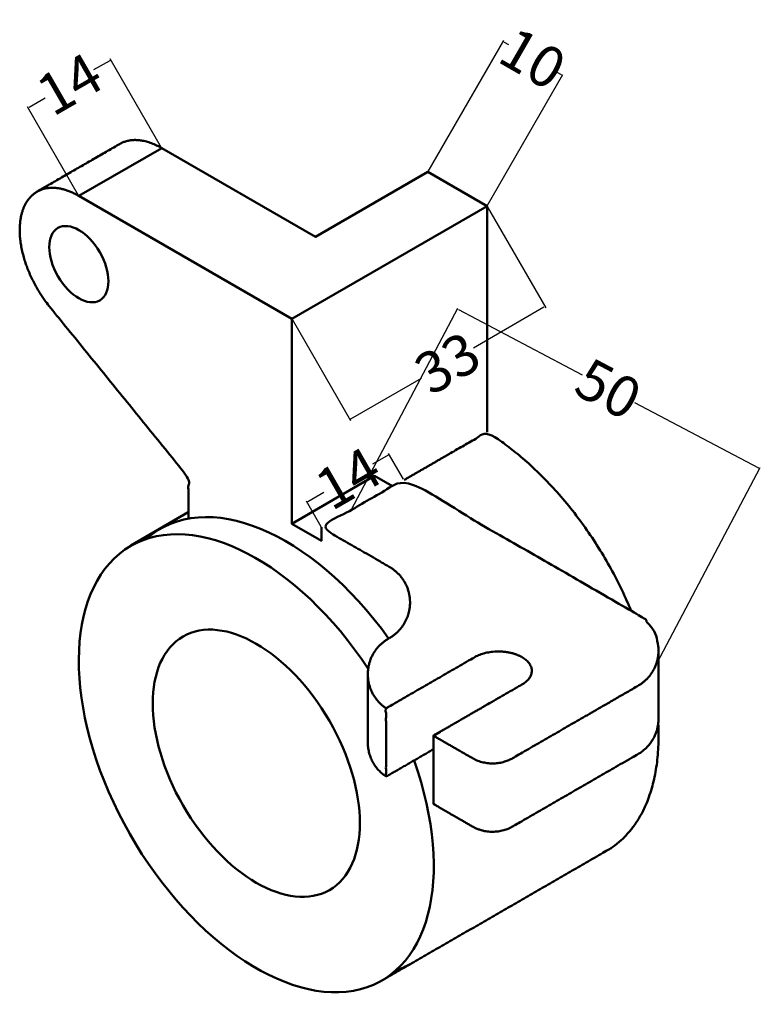
# Model space of a CAD drawing. Units: millimetres. Extents: x -24 to 84, y 4 to 148.
import ezdxf

# ---------------------------------------------------------------- set-up
doc = ezdxf.new("R2010")
doc.units = ezdxf.units.MM
doc.header["$MEASUREMENT"] = 0
doc.layers.add('M-DIMS', color=2, linetype='Continuous', lineweight=25)
doc.layers.add('M-OUTL', color=7, linetype='Continuous', lineweight=50)
doc.styles.get("Standard").update_dxf_attribs({"font": 'arial.ttf'})
doc.dimstyles.get("Standard").update_dxf_attribs({"dimtxt": 6, "dimasz": 0.18, "dimexe": 0.18, "dimexo": 0.0625, "dimgap": 0.09, "dimtad": 0, "dimtoh": 1, "dimdec": 0, "dimzin": 0, "dimdsep": 46, "dimtxsty": 'Standard', "dimcen": 0.09, "dimadec": 0, "dimazin": 0, "dimtfac": 1, "dimtdec": 0, "dimtofl": 0, "dimtmove": 0, "dimatfit": 3, "dimfxl": 1, "dimtolj": 1, "dimtzin": 0, "dimarcsym": 0})

# ---------------------------------------------------------------- blocks, each defined once
blk = doc.blocks.new('*D1')
at = {"layer": 'Defpoints', "color": 0, "transparency": 16777216}
for p in [(55.36, 140.02), (35.67, 125.91), (44.33, 120.91)]:
    blk.add_point(p, dxfattribs=at)
at = {"layer": 'M-DIMS', "color": 0, "lineweight": -2, "transparency": 16777216}
for p, q in [((35.7, 125.96), (46.79, 145.18)), ((46.86, 144.93), (47.49, 144.57)), ((44.36, 120.96), (55.45, 140.18)), ((55.21, 140.11), (54.58, 140.48))]:
    blk.add_line(p, q, dxfattribs=at)
at = {"layer": 'M-DIMS', "color": 0, "transparency": 16777216}
for points in [[(46.87, 144.96), (46.84, 144.91), (46.7, 145.02)], [(55.22, 140.14), (55.19, 140.09), (55.36, 140.02)]]:
    blk.add_solid(points, dxfattribs=at)
at = {"layer": 'M-DIMS', "color": 0, "transparency": 16777216, "insert": (51.03, 142.52), "char_height": 6, "attachment_point": 5, "rotation": 330}
blk.add_mtext('\\A1;10', dxfattribs=at)
blk = doc.blocks.new('*D2')
at = {"layer": 'Defpoints', "color": 0, "transparency": 16777216}
for p in [(44.33, 120.91), (52.83, 106.19), (15.75, 104.41)]:
    blk.add_point(p, dxfattribs=at)
at = {"layer": 'M-DIMS', "color": 0, "lineweight": -2, "transparency": 16777216}
for p, q in [((44.36, 120.86), (52.92, 106.03)), ((52.67, 106.1), (42.34, 100.13)), ((15.78, 104.36), (24.34, 89.53)), ((24.41, 89.78), (34.74, 95.74))]:
    blk.add_line(p, q, dxfattribs=at)
at = {"layer": 'M-DIMS', "color": 0, "transparency": 16777216}
for points in [[(52.66, 106.12), (52.69, 106.07), (52.83, 106.19)], [(24.39, 89.8), (24.42, 89.75), (24.25, 89.69)]]:
    blk.add_solid(points, dxfattribs=at)
at = {"layer": 'M-DIMS', "color": 0, "transparency": 16777216, "insert": (38.54, 97.94), "char_height": 6, "attachment_point": 5, "rotation": 30}
blk.add_mtext('\\A1;33', dxfattribs=at)
blk = doc.blocks.new('*D3')
at = {"layer": 'Defpoints', "color": 0, "transparency": 16777216}
for p in [(-10.74, 142.29), (-3.3, 129.41), (-15.43, 122.41)]:
    blk.add_point(p, dxfattribs=at)
at = {"layer": 'M-DIMS', "color": 0, "lineweight": -2, "transparency": 16777216}
for p, q in [((-10.9, 142.2), (-13.26, 140.84)), ((-3.33, 129.46), (-10.83, 142.45)), ((-22.71, 135.38), (-20.35, 136.75)), ((-15.46, 122.46), (-22.96, 135.45))]:
    blk.add_line(p, q, dxfattribs=at)
at = {"layer": 'M-DIMS', "color": 0, "transparency": 16777216}
for points in [[(-10.91, 142.23), (-10.88, 142.18), (-10.74, 142.29)], [(-22.72, 135.41), (-22.69, 135.36), (-22.87, 135.29)]]:
    blk.add_solid(points, dxfattribs=at)
at = {"layer": 'M-DIMS', "color": 0, "transparency": 16777216, "insert": (-16.8, 138.79), "char_height": 6, "attachment_point": 5, "rotation": 30}
blk.add_mtext('\\A1;14', dxfattribs=at)
blk = doc.blocks.new('*D4')
at = {"layer": 'Defpoints', "color": 0, "transparency": 16777216}
for p in [(30.02, 84.53), (32.14, 80.87), (20.08, 73.91)]:
    blk.add_point(p, dxfattribs=at)
at = {"layer": 'M-DIMS', "color": 0, "lineweight": -2, "transparency": 16777216}
for p, q in [((29.87, 84.44), (27.54, 83.1)), ((32.11, 80.93), (29.93, 84.69)), ((18.12, 77.66), (20.45, 79)), ((20.05, 73.96), (17.88, 77.72))]:
    blk.add_line(p, q, dxfattribs=at)
at = {"layer": 'M-DIMS', "color": 0, "transparency": 16777216}
for points in [[(29.85, 84.47), (29.88, 84.41), (30.02, 84.53)], [(18.11, 77.69), (18.14, 77.63), (17.97, 77.57)]]:
    blk.add_solid(points, dxfattribs=at)
at = {"layer": 'M-DIMS', "color": 0, "transparency": 16777216, "insert": (24, 81.05), "char_height": 6, "attachment_point": 5, "rotation": 30}
blk.add_mtext('\\A1;14', dxfattribs=at)
blk = doc.blocks.new('*D5')
at = {"layer": 'Defpoints', "color": 0, "transparency": 16777216}
for p in [(84.25, 82.46), (24.46, 76.44), (68.74, 53.07)]:
    blk.add_point(p, dxfattribs=at)
at = {"layer": 'M-DIMS', "color": 0, "lineweight": -2, "transparency": 16777216}
for p, q in [((24.49, 76.49), (40.05, 105.99)), ((40.13, 105.75), (58.24, 96.19)), ((84.1, 82.55), (65.98, 92.1)), ((68.77, 53.13), (84.34, 82.62))]:
    blk.add_line(p, q, dxfattribs=at)
at = {"layer": 'M-DIMS', "color": 0, "transparency": 16777216}
for points in [[(40.14, 105.77), (40.12, 105.72), (39.97, 105.83)], [(84.11, 82.57), (84.08, 82.52), (84.25, 82.46)]]:
    blk.add_solid(points, dxfattribs=at)
at = {"layer": 'M-DIMS', "color": 0, "transparency": 16777216, "insert": (62.11, 94.15), "char_height": 6, "attachment_point": 5, "rotation": 332.1791}
blk.add_mtext('\\A1;50', dxfattribs=at)

msp = doc.modelspace()

# ---------------------------------------------------------------- linework, layer by layer
at = {"layer": 'M-OUTL'}
for p, q in [((-7.82, 71.23), (0.59, 76.09)), ((20.08, 73.83), (20.01, 73.87)), ((26.29, 70.25), (26.29, 70.25))]:
    msp.add_line(p, q, dxfattribs=at)
for points in [[(15.75, 104.41), (-15.43, 122.41), (-3.3, 129.41), (19.21, 116.41), (35.67, 125.91), (44.33, 120.91), (44.33, 87.82)], [(44.33, 120.91), (15.75, 104.41), (15.75, 94.41), (15.75, 100.41)], [(30.47, 79.91), (27.87, 81.41), (15.75, 74.41), (15.75, 94.41)], [(20.08, 73.91), (20.08, 71.91), (15.75, 74.41)], [(26.88, 42.43), (26.89, 42.67), (26.89, 52.44)], [(37.47, 43.95), (36.47, 43.37), (36.47, 33.37)]]:
    msp.add_lwpolyline(points, dxfattribs=at)
for centre, major_axis in [((-15.43, 112.41), (3.06, -5.3)), ((10.55, 39.33), (10.72, -18.56))]:
    msp.add_ellipse(centre, major_axis=major_axis, ratio=0.57735, dxfattribs=at)
for centre, start_param, end_param in [((14.88, 41.83), 1.738401, 3.259718), ((10.55, 39.33), 1.674147, 7.54448), ((43.46, 58.33), 5.225411, 5.238866), ((14.88, 41.83), 6.16506, 6.283185)]:
    msp.add_ellipse(centre, major_axis=(18.37, -31.82), ratio=0.57735, start_param=start_param, end_param=end_param, dxfattribs=at)
for points, weights, knots in [([(-3.3, 129.41), (-6.89, 131.48), (-9.43, 130.02), (-15.49, 126.52), (-21.55, 123.02)], [1, 0.923879532511, 1, 1, 1], [0, 0, 0, 0.785398, 0.785398, 1.785398, 1.785398, 1.785398]), ([(-15.43, 122.41), (-22.1, 126.26), (-23.8, 119.79), (-25.5, 113.33), (-19.7, 106.18), (-9.54, 93.66), (0.62, 81.14), (0.62, 78.14), (0.62, 75.14)], [1, 0.792142227149, 1, 0.792142227149, 1, 1, 1, 1, 1], [0, 0, 0, 1.312971, 1.312971, 2.625941, 2.625941, 3.625941, 3.625941, 4.625941, 4.625941, 4.625941]), ([(65.44, 61.64), (58.09, 79.34), (44.33, 87.82), (38.27, 84.32), (32.22, 80.82)], [1, 0.883525266663, 1, 1, 1], [0, 0, 0, 0.974921, 0.974921, 1.974921, 1.974921, 1.974921]), ([(36.47, 41.37), (33.01, 39.37), (29.54, 37.37), (29.54, 42.37), (29.54, 47.37), (36.03, 51.12), (42.53, 54.87), (44.53, 56.03), (47.26, 55.6), (49.99, 55.18), (50.72, 53.6), (51.46, 52.03), (49.46, 50.87), (42.96, 47.12), (36.47, 43.37), (39.3, 41.74), (42.13, 40.1), (45.13, 38.37), (48.13, 40.1), (57.28, 45.39), (66.44, 50.67), (69.44, 52.41), (69.44, 55.87), (69.44, 59.34), (66.44, 61.07), (49.29, 70.97), (32.14, 80.87), (26.07, 77.37), (20.01, 73.87), (25.04, 70.97), (30.06, 68.07), (33.06, 66.34), (33.06, 62.87), (33.06, 59.41), (30.06, 57.67), (29.97, 57.62), (29.88, 57.57), (26.88, 55.84), (26.88, 52.37), (26.88, 49.15), (29.56, 47.37)], [1, 1, 1, 1, 1, 1, 1, 0.866025403784, 1, 0.866025403784, 1, 0.866025403784, 1, 1, 1, 1, 1, 0.866025403784, 1, 1, 1, 0.866025403784, 1, 0.866025403784, 1, 1, 1, 1, 1, 1, 1, 0.866025403784, 1, 0.866025403784, 1, 1, 1, 0.866025403784, 1, 0.874277463381, 0.984512439012], [0, 0, 0, 0.5338, 0.5338, 1.5338, 1.5338, 2.5338, 2.5338, 3.580998, 3.580998, 4.628195, 4.628195, 5.675393, 5.675393, 6.675393, 6.675393, 7.675393, 7.675393, 8.72259, 8.72259, 9.72259, 9.72259, 10.769788, 10.769788, 11.816985, 11.816985, 12.816985, 12.816985, 13.816985, 13.816985, 14.816985, 14.816985, 15.864183, 15.864183, 16.91138, 16.91138, 17.91138, 17.91138, 18.958578, 18.958578, 19.941274, 19.941274, 19.941274]), ([(69.44, 55.87), (69.44, 50.91), (69.44, 45.94), (69.44, 45.91), (69.44, 45.87), (69.44, 42.41), (66.44, 40.67), (57.28, 35.39), (48.13, 30.1), (45.13, 28.37), (42.13, 30.1), (39.3, 31.74), (36.47, 33.37)], [1, 1, 1, 0.99839585123, 1, 0.866025403784, 1, 1, 1, 0.866025403784, 1, 1, 1], [0, 0, 0, 1, 1, 1.012539, 1.012539, 2.059736, 2.059736, 3.059736, 3.059736, 4.106934, 4.106934, 5.106934, 5.106934, 5.106934]), ([(29.54, 47.36), (29.7, 47.47), (29.88, 47.57), (29.97, 47.62), (30.06, 47.67)], [0.983447338978, 0.991137396037, 1, 1, 1], [2.025122, 2.025122, 2.025122, 2.094395, 2.094395, 3.094395, 3.094395, 3.094395]), ([(28.92, 7.51), (45.38, 17.01), (61.83, 26.51), (70.1, 31.28), (69.4, 45.16)], [1, 1, 1, 0.911954175248, 1], [0, 0, 0, 1, 1, 1.845549, 1.845549, 1.845549]), ([(29.55, 37.38), (26.88, 39.16), (26.88, 42.37), (26.88, 42.52), (26.89, 42.67)], [0.984016292634, 0.874561074562, 1, 0.993335156546, 0.987333425944], [0.066718, 0.066718, 0.066718, 1.047198, 1.047198, 1.099293, 1.099293, 1.099293])]:
    msp.add_rational_spline(points, weights, degree=2, knots=knots, dxfattribs=at)
msp.add_open_spline([(48.13, 40.1), (48.79, 40.49), (49.46, 40.87)], degree=2, dxfattribs=at)

# ---------------------------------------------------------------- dimensions: what is measured, and where the dimension line sits
at = {"layer": 'M-DIMS'}
for p1, p2, distance, picture, middle in [((35.67, 125.91), (44.33, 120.91), 22.07, '*D1', (51.03, 142.52)), ((-15.43, 122.41), (-3.3, 129.41), 14.88, '*D3', (-16.8, 138.79)), ((15.75, 104.41), (44.33, 120.91), -17, '*D2', (38.54, 97.94)), ((24.46, 76.44), (68.74, 53.07), 33.23, '*D5', (62.11, 94.15)), ((20.08, 73.91), (32.14, 80.87), 4.23, '*D4', (24, 81.05))]:
    dim = msp.add_aligned_dim(p1=p1, p2=p2, distance=distance, dimstyle='Standard', override={"dimclrd": 0, "dimclre": 0, "dimclrt": 0}, dxfattribs=at)
    dim.commit()
    dim.dimension.update_dxf_attribs({"geometry": picture, "text_midpoint": middle})

doc.saveas('drawing.dxf')
